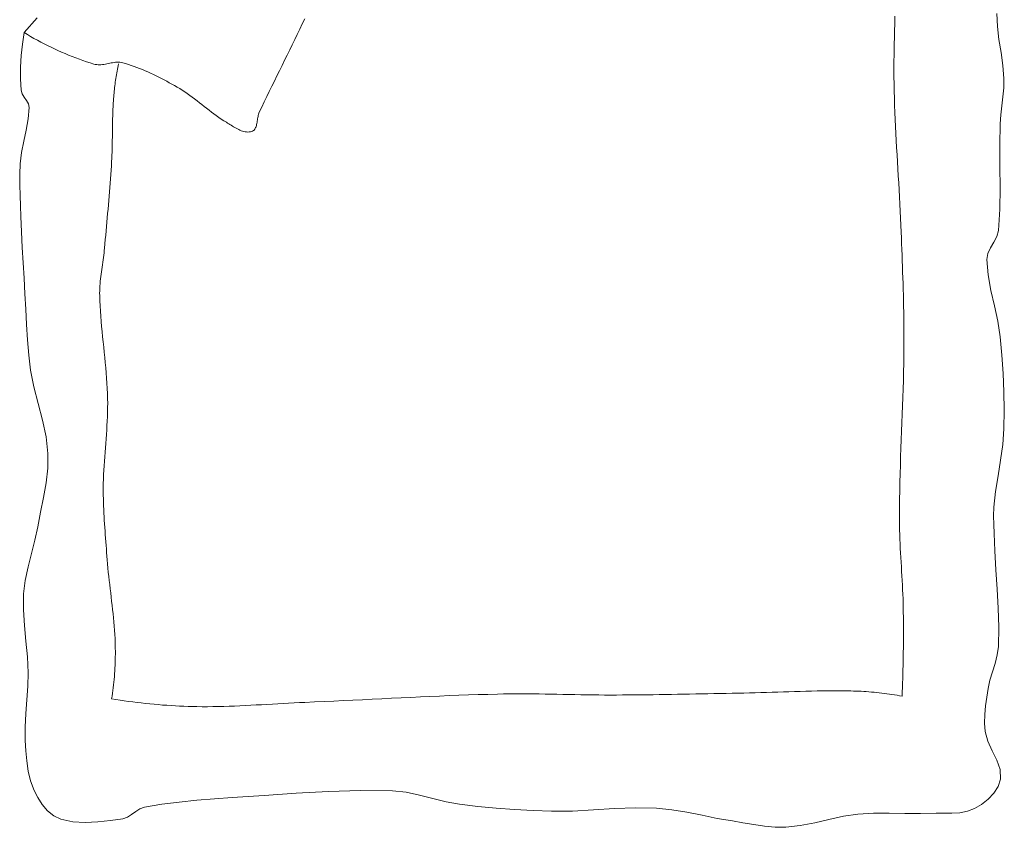
# Model space of a CAD drawing. Units: inches. Extents: x -36302355 to 648, y -221479757 to 75.
# Tile 32 of 37: x 284 to 340, y -66 to -20. Entities that reach past the tile are written whole.
import ezdxf

# ---------------------------------------------------------------- set-up
doc = ezdxf.new("R2010")
doc.units = ezdxf.units.IN
doc.header["$MEASUREMENT"] = 0
doc.layers.add('A-FURN', color=8, linetype='Continuous', lineweight=13)

# ---------------------------------------------------------------- blocks, each defined once
blk = doc.blocks.new('BED-DOUBLE')
for p, q in [((1, 46.159), (0.249, 45.317)), ((16.116, 45.81), (16.256, 46.108)), ((49.913, 45.995), (49.92, 46.246)), ((55.763, 45.66), (55.733, 46.404)), ((15.832, 45.216), (15.975, 45.513)), ((15.975, 45.513), (16.116, 45.81)), ((49.893, 45.241), (49.899, 45.492)), ((49.899, 45.492), (49.906, 45.743)), ((49.906, 45.743), (49.913, 45.995)), ((55.854, 44.918), (55.763, 45.66)), ((0.249, 45.317), (0.154, 44.664)), ((0.249, 45.317), (0.437, 45.204)), ((0.437, 45.204), (0.625, 45.093)), ((0.625, 45.093), (0.815, 44.985)), ((0.815, 44.985), (1.007, 44.879)), ((15.689, 44.919), (15.832, 45.216)), ((49.881, 44.738), (49.887, 44.989)), ((49.887, 44.989), (49.893, 45.241)), ((0.154, 44.664), (0.089, 44.006)), ((1.007, 44.879), (1.2, 44.776)), ((1.2, 44.776), (1.394, 44.675)), ((1.394, 44.675), (1.59, 44.576)), ((1.59, 44.576), (1.787, 44.479)), ((1.787, 44.479), (1.985, 44.386)), ((1.985, 44.386), (2.185, 44.294)), ((15.4, 44.327), (15.545, 44.623)), ((15.545, 44.623), (15.689, 44.919)), ((49.872, 44.235), (49.876, 44.487)), ((49.876, 44.487), (49.881, 44.738)), ((55.971, 44.178), (55.854, 44.918)), ((0.089, 44.006), (0.055, 43.345)), ((2.185, 44.294), (2.385, 44.205)), ((2.385, 44.205), (2.587, 44.119)), ((2.587, 44.119), (2.789, 44.035)), ((2.789, 44.035), (2.993, 43.954)), ((2.993, 43.954), (3.198, 43.875)), ((3.198, 43.875), (3.403, 43.799)), ((15.109, 43.736), (15.255, 44.031)), ((15.255, 44.031), (15.4, 44.327)), ((49.866, 43.733), (49.868, 43.984)), ((49.868, 43.984), (49.872, 44.235)), ((56.076, 43.436), (55.971, 44.178)), ((0.055, 43.345), (0.053, 42.684)), ((3.403, 43.799), (3.609, 43.726)), ((3.609, 43.726), (3.816, 43.655)), ((3.816, 43.655), (4.024, 43.587)), ((4.024, 43.587), (4.233, 43.522)), ((4.233, 43.522), (4.312, 43.502)), ((4.312, 43.502), (4.392, 43.489)), ((4.392, 43.489), (4.473, 43.482)), ((4.473, 43.482), (4.554, 43.482)), ((4.554, 43.482), (4.636, 43.486)), ((4.636, 43.486), (4.719, 43.494)), ((4.719, 43.494), (4.802, 43.505)), ((4.802, 43.505), (4.885, 43.519)), ((4.885, 43.519), (4.969, 43.535)), ((4.969, 43.535), (5.052, 43.552)), ((5.052, 43.552), (5.136, 43.569)), ((5.136, 43.569), (5.22, 43.585)), ((5.22, 43.585), (5.303, 43.599)), ((5.303, 43.599), (5.386, 43.611)), ((5.386, 43.611), (5.469, 43.621)), ((5.469, 43.621), (5.552, 43.626)), ((5.552, 43.626), (5.634, 43.627)), ((5.594, 43.326), (5.575, 43.223)), ((5.615, 43.43), (5.594, 43.326)), ((5.636, 43.533), (5.615, 43.43)), ((5.634, 43.627), (5.715, 43.622)), ((5.715, 43.622), (5.795, 43.611)), ((5.795, 43.611), (5.875, 43.593)), ((5.875, 43.593), (6.038, 43.546)), ((6.038, 43.546), (6.201, 43.496)), ((6.201, 43.496), (6.362, 43.443)), ((6.362, 43.443), (6.523, 43.387)), ((6.523, 43.387), (6.683, 43.329)), ((6.683, 43.329), (6.841, 43.268)), ((6.841, 43.268), (6.999, 43.204)), ((14.817, 43.145), (14.963, 43.44)), ((14.963, 43.44), (15.109, 43.736)), ((49.863, 43.23), (49.864, 43.481)), ((49.864, 43.481), (49.866, 43.733)), ((56.134, 42.692), (56.076, 43.436)), ((0.053, 42.684), (0.081, 42.025)), ((5.486, 42.703), (5.47, 42.599)), ((5.502, 42.808), (5.486, 42.703)), ((5.519, 42.912), (5.502, 42.808)), ((5.537, 43.015), (5.519, 42.912)), ((5.555, 43.119), (5.537, 43.015)), ((5.575, 43.223), (5.555, 43.119)), ((6.999, 43.204), (7.157, 43.138)), ((7.157, 43.138), (7.313, 43.07)), ((7.313, 43.07), (7.468, 43)), ((7.468, 43), (7.623, 42.928)), ((7.623, 42.928), (7.777, 42.854)), ((7.777, 42.854), (7.93, 42.778)), ((7.93, 42.778), (8.082, 42.701)), ((8.082, 42.701), (8.234, 42.622)), ((14.526, 42.554), (14.672, 42.849)), ((14.672, 42.849), (14.817, 43.145)), ((49.863, 42.979), (49.863, 43.23)), ((49.865, 42.727), (49.863, 42.979)), ((49.868, 42.476), (49.865, 42.727)), ((56.124, 42.175), (56.134, 42.692)), ((5.415, 42.181), (5.403, 42.077)), ((5.428, 42.286), (5.415, 42.181)), ((5.441, 42.39), (5.428, 42.286)), ((5.455, 42.495), (5.441, 42.39)), ((5.47, 42.599), (5.455, 42.495)), ((8.234, 42.622), (8.384, 42.542)), ((8.384, 42.542), (8.534, 42.46)), ((8.534, 42.46), (8.683, 42.378)), ((8.683, 42.378), (8.832, 42.295)), ((8.832, 42.295), (8.98, 42.21)), ((8.98, 42.21), (9.128, 42.123)), ((9.128, 42.123), (9.274, 42.031)), ((14.237, 41.962), (14.381, 42.258)), ((14.381, 42.258), (14.526, 42.554)), ((49.872, 42.225), (49.868, 42.476)), ((49.878, 41.973), (49.872, 42.225)), ((56.078, 41.659), (56.124, 42.175)), ((0.081, 42.025), (0.139, 41.819)), ((0.139, 41.819), (0.255, 41.628)), ((0.255, 41.628), (0.387, 41.441)), ((5.362, 41.657), (5.353, 41.552)), ((5.371, 41.762), (5.362, 41.657)), ((5.381, 41.867), (5.371, 41.762)), ((5.392, 41.972), (5.381, 41.867)), ((5.403, 42.077), (5.392, 41.972)), ((9.274, 42.031), (9.418, 41.936)), ((9.418, 41.936), (9.561, 41.838)), ((9.561, 41.838), (9.701, 41.738)), ((9.701, 41.738), (9.84, 41.635)), ((9.84, 41.635), (9.978, 41.531)), ((13.95, 41.369), (14.093, 41.666)), ((14.093, 41.666), (14.237, 41.962)), ((49.889, 41.571), (49.878, 41.973)), ((49.903, 41.169), (49.889, 41.571)), ((56.015, 41.144), (56.078, 41.659)), ((0.387, 41.441), (0.496, 41.249)), ((0.54, 41.043), (0.489, 40.398)), ((0.496, 41.249), (0.54, 41.043)), ((5.325, 41.1), (5.317, 40.926)), ((5.334, 41.274), (5.325, 41.1)), ((5.346, 41.447), (5.334, 41.274)), ((5.353, 41.552), (5.346, 41.447)), ((9.978, 41.531), (10.115, 41.425)), ((10.115, 41.425), (10.252, 41.319)), ((10.252, 41.319), (10.388, 41.212)), ((10.388, 41.212), (10.524, 41.105)), ((10.524, 41.105), (10.661, 40.998)), ((10.661, 40.998), (10.798, 40.892)), ((13.668, 40.774), (13.808, 41.071)), ((13.808, 41.071), (13.95, 41.369)), ((49.918, 40.767), (49.903, 41.169)), ((55.955, 40.628), (56.015, 41.144)), ((5.305, 40.579), (5.301, 40.405)), ((5.311, 40.753), (5.305, 40.579)), ((5.317, 40.926), (5.311, 40.753)), ((10.798, 40.892), (10.935, 40.786)), ((10.935, 40.786), (11.074, 40.683)), ((11.074, 40.683), (11.213, 40.581)), ((11.213, 40.581), (11.354, 40.481)), ((11.354, 40.481), (11.497, 40.385)), ((13.57, 40.401), (13.581, 40.468)), ((13.581, 40.468), (13.594, 40.534)), ((13.594, 40.534), (13.608, 40.598)), ((13.608, 40.598), (13.625, 40.659)), ((13.625, 40.659), (13.645, 40.718)), ((13.645, 40.718), (13.668, 40.774)), ((49.935, 40.364), (49.918, 40.767)), ((55.918, 40.112), (55.955, 40.628)), ((0.489, 40.398), (0.377, 39.758)), ((5.293, 39.883), (5.291, 39.709)), ((5.295, 40.057), (5.293, 39.883)), ((5.298, 40.231), (5.295, 40.057)), ((5.301, 40.405), (5.298, 40.231)), ((11.497, 40.385), (11.642, 40.291)), ((11.642, 40.291), (11.789, 40.201)), ((11.789, 40.201), (11.856, 40.16)), ((11.856, 40.16), (11.923, 40.118)), ((11.923, 40.118), (11.991, 40.075)), ((11.991, 40.075), (12.061, 40.031)), ((12.061, 40.031), (12.131, 39.988)), ((12.131, 39.988), (12.201, 39.944)), ((12.201, 39.944), (12.273, 39.902)), ((12.273, 39.902), (12.345, 39.86)), ((13.433, 39.847), (13.458, 39.897)), ((13.458, 39.897), (13.48, 39.952)), ((13.48, 39.952), (13.498, 40.01)), ((13.498, 40.01), (13.513, 40.071)), ((13.513, 40.071), (13.527, 40.135)), ((13.527, 40.135), (13.539, 40.2)), ((13.539, 40.2), (13.549, 40.267)), ((13.549, 40.267), (13.56, 40.334)), ((13.56, 40.334), (13.57, 40.401)), ((49.954, 39.962), (49.935, 40.364)), ((49.974, 39.56), (49.954, 39.962)), ((55.898, 38.895), (55.918, 40.112)), ((0.377, 39.758), (0.24, 39.119)), ((5.287, 39.361), (5.284, 39.187)), ((5.289, 39.535), (5.287, 39.361)), ((5.291, 39.709), (5.289, 39.535)), ((12.345, 39.86), (12.418, 39.821)), ((12.418, 39.821), (12.491, 39.785)), ((12.491, 39.785), (12.564, 39.752)), ((12.564, 39.752), (12.638, 39.722)), ((12.638, 39.722), (12.712, 39.696)), ((12.712, 39.696), (12.786, 39.675)), ((12.786, 39.675), (12.86, 39.659)), ((12.86, 39.659), (12.934, 39.649)), ((12.934, 39.649), (13.008, 39.646)), ((13.008, 39.646), (13.082, 39.649)), ((13.082, 39.649), (13.156, 39.659)), ((13.156, 39.659), (13.229, 39.677)), ((13.229, 39.677), (13.282, 39.698)), ((13.282, 39.698), (13.328, 39.726)), ((13.328, 39.726), (13.369, 39.761)), ((13.369, 39.761), (13.403, 39.801)), ((13.403, 39.801), (13.433, 39.847)), ((49.996, 39.159), (49.974, 39.56)), ((0.24, 39.119), (0.112, 38.48)), ((5.278, 38.839), (5.274, 38.666)), ((5.282, 39.013), (5.278, 38.839)), ((5.284, 39.187), (5.282, 39.013)), ((50.018, 38.757), (49.996, 39.159)), ((50.04, 38.355), (50.018, 38.757)), ((55.907, 37.677), (55.898, 38.895)), ((0.112, 38.48), (0.028, 37.836)), ((5.262, 38.318), (5.254, 38.144)), ((5.268, 38.492), (5.262, 38.318)), ((5.274, 38.666), (5.268, 38.492)), ((50.064, 37.953), (50.04, 38.355)), ((0.028, 37.836), (0, 37.235)), ((5.229, 37.723), (5.213, 37.476)), ((5.244, 37.971), (5.229, 37.723)), ((5.254, 38.144), (5.244, 37.971)), ((50.087, 37.551), (50.064, 37.953)), ((55.917, 36.459), (55.907, 37.677)), ((0, 37.235), (0, 36.634)), ((5.196, 37.228), (5.178, 36.981)), ((5.213, 37.476), (5.196, 37.228)), ((50.111, 37.149), (50.087, 37.551)), ((50.134, 36.747), (50.111, 37.149)), ((0, 36.634), (0.018, 36.032)), ((5.159, 36.734), (5.14, 36.487)), ((5.178, 36.981), (5.159, 36.734)), ((50.157, 36.345), (50.134, 36.747)), ((0.018, 36.032), (0.045, 35.43)), ((5.1, 35.992), (5.08, 35.745)), ((5.12, 36.239), (5.1, 35.992)), ((5.14, 36.487), (5.12, 36.239)), ((50.179, 35.943), (50.157, 36.345)), ((50.201, 35.542), (50.179, 35.943)), ((55.897, 35.242), (55.917, 36.459)), ((0.045, 35.43), (0.071, 34.828)), ((5.058, 35.498), (5.037, 35.251)), ((5.08, 35.745), (5.058, 35.498)), ((50.222, 35.14), (50.201, 35.542)), ((0.071, 34.828), (0.107, 33.948)), ((5.015, 35.004), (4.993, 34.757)), ((5.037, 35.251), (5.015, 35.004)), ((50.241, 34.737), (50.222, 35.14)), ((55.818, 34.029), (55.897, 35.242)), ((4.949, 34.263), (4.926, 34.016)), ((4.971, 34.51), (4.949, 34.263)), ((4.993, 34.757), (4.971, 34.51)), ((50.259, 34.335), (50.241, 34.737)), ((50.275, 33.933), (50.259, 34.335)), ((0.107, 33.948), (0.149, 33.068)), ((4.904, 33.769), (4.882, 33.522)), ((4.926, 34.016), (4.904, 33.769)), ((50.287, 33.608), (50.275, 33.933)), ((55.726, 33.689), (55.818, 34.029)), ((4.859, 33.275), (4.837, 33.028)), ((4.882, 33.522), (4.859, 33.275)), ((50.3, 33.282), (50.287, 33.608)), ((50.312, 32.957), (50.3, 33.282)), ((55.37, 33.05), (55.558, 33.367)), ((55.558, 33.367), (55.726, 33.689)), ((0.149, 33.068), (0.196, 32.188)), ((4.793, 32.623), (4.776, 32.487)), ((4.809, 32.758), (4.793, 32.623)), ((4.824, 32.893), (4.809, 32.758)), ((4.837, 33.028), (4.824, 32.893)), ((50.325, 32.632), (50.312, 32.957)), ((50.337, 32.306), (50.325, 32.632)), ((55.16, 32.385), (55.219, 32.726)), ((55.219, 32.726), (55.37, 33.05)), ((0.196, 32.188), (0.247, 31.308)), ((4.719, 32.082), (4.7, 31.947)), ((4.739, 32.217), (4.719, 32.082)), ((4.758, 32.352), (4.739, 32.217)), ((4.776, 32.487), (4.758, 32.352)), ((50.348, 31.981), (50.337, 32.306)), ((55.234, 31.495), (55.16, 32.385)), ((4.644, 31.542), (4.627, 31.407)), ((4.662, 31.677), (4.644, 31.542)), ((4.681, 31.812), (4.662, 31.677)), ((4.7, 31.947), (4.681, 31.812)), ((50.36, 31.655), (50.348, 31.981)), ((50.371, 31.33), (50.36, 31.655)), ((55.394, 30.613), (55.234, 31.495)), ((0.247, 31.308), (0.302, 30.429)), ((4.586, 31.001), (4.576, 30.866)), ((4.598, 31.136), (4.586, 31.001)), ((4.612, 31.272), (4.598, 31.136)), ((4.627, 31.407), (4.612, 31.272)), ((50.381, 31.004), (50.371, 31.33)), ((50.39, 30.679), (50.381, 31.004)), ((0.302, 30.429), (0.351, 29.554)), ((4.563, 30.595), (4.561, 30.459)), ((4.561, 30.459), (4.562, 30.323)), ((4.568, 30.73), (4.563, 30.595)), ((4.576, 30.866), (4.568, 30.73)), ((50.399, 30.353), (50.39, 30.679)), ((50.408, 30.028), (50.399, 30.353)), ((55.593, 29.734), (55.394, 30.613)), ((4.562, 30.323), (4.57, 30.028)), ((4.57, 30.028), (4.583, 29.734)), ((50.415, 29.702), (50.408, 30.028)), ((0.351, 29.554), (0.396, 28.679)), ((4.583, 29.734), (4.601, 29.439)), ((4.601, 29.439), (4.621, 29.145)), ((50.421, 29.376), (50.415, 29.702)), ((50.426, 29.051), (50.421, 29.376)), ((55.784, 28.854), (55.593, 29.734)), ((0.396, 28.679), (0.448, 27.804)), ((4.621, 29.145), (4.645, 28.851)), ((4.645, 28.851), (4.671, 28.557)), ((50.43, 28.725), (50.426, 29.051)), ((50.433, 28.4), (50.43, 28.725)), ((55.919, 27.967), (55.784, 28.854)), ((4.671, 28.557), (4.699, 28.263)), ((4.699, 28.263), (4.728, 27.969)), ((50.435, 28.074), (50.433, 28.4)), ((0.448, 27.804), (0.521, 26.932)), ((4.728, 27.969), (4.759, 27.675)), ((4.759, 27.675), (4.79, 27.382)), ((50.434, 27.423), (50.435, 27.749)), ((50.435, 27.749), (50.435, 28.074)), ((56.015, 26.923), (55.919, 27.967)), ((4.79, 27.382), (4.821, 27.088)), ((4.821, 27.088), (4.852, 26.794)), ((50.429, 26.939), (50.434, 27.423)), ((0.521, 26.932), (0.625, 26.063)), ((4.852, 26.794), (4.881, 26.5)), ((4.881, 26.5), (4.909, 26.207)), ((50.412, 25.97), (50.422, 26.454)), ((50.422, 26.454), (50.429, 26.939)), ((56.091, 25.876), (56.015, 26.923)), ((0.625, 26.063), (0.809, 25.109)), ((4.909, 26.207), (4.935, 25.913)), ((4.935, 25.913), (4.958, 25.618)), ((50.399, 25.486), (50.412, 25.97)), ((56.14, 24.828), (56.091, 25.876)), ((4.958, 25.618), (4.978, 25.324)), ((4.978, 25.324), (4.995, 25.03)), ((50.385, 25.001), (50.399, 25.486)), ((0.809, 25.109), (1.05, 24.163)), ((4.995, 25.03), (5.007, 24.735)), ((5.007, 24.735), (5.015, 24.44)), ((50.37, 24.517), (50.385, 25.001)), ((56.158, 23.779), (56.14, 24.828)), ((1.05, 24.163), (1.298, 23.22)), ((5.015, 24.44), (5.018, 24.185)), ((5.018, 24.185), (5.016, 23.931)), ((50.353, 24.033), (50.37, 24.517)), ((5.011, 23.676), (5.002, 23.421)), ((5.016, 23.931), (5.011, 23.676)), ((50.336, 23.549), (50.353, 24.033)), ((56.139, 22.73), (56.158, 23.779)), ((1.298, 23.22), (1.501, 22.271)), ((4.991, 23.166), (4.977, 22.912)), ((5.002, 23.421), (4.991, 23.166)), ((50.299, 22.581), (50.317, 23.065)), ((50.317, 23.065), (50.336, 23.549)), ((4.961, 22.657), (4.943, 22.403)), ((4.977, 22.912), (4.961, 22.657)), ((50.281, 22.096), (50.299, 22.581)), ((56.069, 21.831), (56.139, 22.73)), ((1.501, 22.271), (1.61, 21.31)), ((4.924, 22.148), (4.905, 21.894)), ((4.943, 22.403), (4.924, 22.148)), ((50.263, 21.612), (50.281, 22.096)), ((4.866, 21.385), (4.847, 21.13)), ((4.885, 21.639), (4.866, 21.385)), ((4.905, 21.894), (4.885, 21.639)), ((50.245, 21.128), (50.263, 21.612)), ((55.946, 20.936), (56.069, 21.831)), ((1.61, 21.31), (1.596, 20.47)), ((4.829, 20.876), (4.812, 20.621)), ((4.847, 21.13), (4.829, 20.876)), ((50.229, 20.644), (50.245, 21.128)), ((55.8, 20.042), (55.946, 20.936)), ((1.596, 20.47), (1.501, 19.634)), ((4.798, 20.366), (4.785, 20.111)), ((4.812, 20.621), (4.798, 20.366)), ((50.215, 20.16), (50.229, 20.644)), ((4.776, 19.857), (4.77, 19.602)), ((4.785, 20.111), (4.776, 19.857)), ((50.19, 19.191), (50.201, 19.676)), ((50.201, 19.676), (50.215, 20.16)), ((55.663, 19.148), (55.8, 20.042)), ((1.501, 19.634), (1.355, 18.801)), ((4.77, 19.602), (4.767, 19.347)), ((4.767, 19.347), (4.767, 19.142)), ((4.767, 19.142), (4.77, 18.938)), ((50.182, 18.707), (50.19, 19.191)), ((55.566, 18.25), (55.663, 19.148)), ((1.355, 18.801), (1.187, 17.969)), ((4.77, 18.938), (4.773, 18.733)), ((4.773, 18.733), (4.779, 18.528)), ((50.176, 18.223), (50.182, 18.707)), ((4.779, 18.528), (4.786, 18.323)), ((4.786, 18.323), (4.794, 18.119)), ((4.794, 18.119), (4.803, 17.914)), ((50.173, 17.738), (50.176, 18.223)), ((55.546, 17.754), (55.566, 18.25)), ((1.187, 17.969), (1.029, 17.139)), ((4.803, 17.914), (4.814, 17.71)), ((4.814, 17.71), (4.826, 17.505)), ((4.826, 17.505), (4.838, 17.301)), ((50.174, 17.476), (50.173, 17.738)), ((50.177, 17.214), (50.174, 17.476)), ((55.553, 17.258), (55.546, 17.754)), ((1.029, 17.139), (0.867, 16.371)), ((4.838, 17.301), (4.852, 17.096)), ((4.852, 17.096), (4.866, 16.892)), ((4.866, 16.892), (4.88, 16.688)), ((50.183, 16.952), (50.177, 17.214)), ((50.192, 16.69), (50.183, 16.952)), ((55.576, 16.762), (55.553, 17.258)), ((0.867, 16.371), (0.673, 15.608)), ((4.88, 16.688), (4.895, 16.483)), ((4.895, 16.483), (4.911, 16.279)), ((50.202, 16.429), (50.192, 16.69)), ((50.214, 16.167), (50.202, 16.429)), ((55.604, 16.266), (55.576, 16.762)), ((4.911, 16.279), (4.927, 16.075)), ((4.927, 16.075), (4.943, 15.87)), ((4.943, 15.87), (4.959, 15.666)), ((50.227, 15.905), (50.214, 16.167)), ((50.241, 15.643), (50.227, 15.905)), ((55.626, 15.769), (55.604, 16.266)), ((55.678, 14.678), (55.626, 15.769)), ((0.673, 15.608), (0.479, 14.846)), ((4.959, 15.666), (4.975, 15.462)), ((4.975, 15.462), (4.991, 15.258)), ((4.991, 15.258), (5.01, 15.021)), ((50.256, 15.381), (50.241, 15.643)), ((50.272, 15.12), (50.256, 15.381)), ((0.479, 14.846), (0.317, 14.08)), ((5.01, 15.021), (5.032, 14.784)), ((5.032, 14.784), (5.055, 14.547)), ((50.287, 14.858), (50.272, 15.12)), ((50.303, 14.596), (50.287, 14.858)), ((55.747, 13.587), (55.678, 14.678)), ((0.317, 14.08), (0.222, 13.304)), ((5.055, 14.547), (5.08, 14.31)), ((5.08, 14.31), (5.106, 14.074)), ((5.106, 14.074), (5.133, 13.837)), ((50.319, 14.334), (50.303, 14.596)), ((50.333, 14.073), (50.319, 14.334)), ((50.347, 13.811), (50.333, 14.073)), ((5.133, 13.837), (5.161, 13.601)), ((5.161, 13.601), (5.189, 13.364)), ((50.36, 13.549), (50.347, 13.811)), ((50.371, 13.287), (50.36, 13.549)), ((55.809, 12.496), (55.747, 13.587)), ((0.222, 13.304), (0.211, 12.406)), ((5.189, 13.364), (5.218, 13.128)), ((5.218, 13.128), (5.246, 12.892)), ((50.381, 13.025), (50.371, 13.287)), ((50.388, 12.763), (50.381, 13.025)), ((0.211, 12.406), (0.269, 11.508)), ((5.246, 12.892), (5.273, 12.655)), ((5.273, 12.655), (5.3, 12.419)), ((5.3, 12.419), (5.325, 12.182)), ((50.394, 12.501), (50.388, 12.763)), ((50.397, 12.25), (50.394, 12.501)), ((55.842, 11.405), (55.809, 12.496)), ((5.325, 12.182), (5.349, 11.946)), ((5.349, 11.946), (5.372, 11.709)), ((50.4, 11.999), (50.397, 12.25)), ((50.402, 11.747), (50.4, 11.999)), ((0.269, 11.508), (0.358, 10.61)), ((5.372, 11.709), (5.392, 11.472)), ((5.392, 11.472), (5.41, 11.235)), ((5.41, 11.235), (5.425, 10.998)), ((50.403, 11.496), (50.402, 11.747)), ((50.404, 11.244), (50.403, 11.496)), ((50.404, 10.993), (50.404, 11.244)), ((55.821, 10.315), (55.842, 11.405)), ((5.425, 10.998), (5.438, 10.76)), ((5.438, 10.76), (5.447, 10.523)), ((50.402, 10.49), (50.403, 10.742)), ((50.403, 10.742), (50.404, 10.993)), ((0.358, 10.61), (0.444, 9.712)), ((5.447, 10.523), (5.452, 10.363)), ((5.452, 10.363), (5.454, 10.202)), ((5.454, 10.202), (5.456, 10.042)), ((50.397, 9.987), (50.4, 10.239)), ((50.4, 10.239), (50.402, 10.49)), ((55.755, 9.827), (55.821, 10.315)), ((0.444, 9.712), (0.487, 8.812)), ((5.451, 9.56), (5.446, 9.399)), ((5.454, 9.721), (5.451, 9.56)), ((5.456, 9.881), (5.454, 9.721)), ((5.456, 10.042), (5.456, 9.881)), ((50.389, 9.485), (50.393, 9.736)), ((50.393, 9.736), (50.397, 9.987)), ((55.631, 9.348), (55.755, 9.827)), ((5.432, 9.078), (5.422, 8.918)), ((5.44, 9.239), (5.432, 9.078)), ((5.446, 9.399), (5.44, 9.239)), ((50.379, 8.982), (50.384, 9.233)), ((50.384, 9.233), (50.389, 9.485)), ((55.479, 8.873), (55.631, 9.348)), ((0.487, 8.812), (0.469, 8.039)), ((5.385, 8.437), (5.37, 8.278)), ((5.399, 8.598), (5.385, 8.437)), ((5.412, 8.758), (5.399, 8.598)), ((5.422, 8.918), (5.412, 8.758)), ((50.357, 8.228), (50.365, 8.479)), ((50.365, 8.479), (50.372, 8.731)), ((50.372, 8.731), (50.379, 8.982)), ((55.334, 8.396), (55.479, 8.873)), ((0.469, 8.039), (0.415, 7.265)), ((5.335, 7.958), (5.315, 7.799)), ((5.353, 8.118), (5.335, 7.958)), ((5.37, 8.278), (5.353, 8.118)), ((50.34, 7.726), (50.349, 7.977)), ((50.349, 7.977), (50.357, 8.228)), ((55.153, 7.423), (55.228, 7.912)), ((55.228, 7.912), (55.334, 8.396)), ((5.27, 7.481), (5.246, 7.323)), ((5.246, 7.323), (5.486, 7.284)), ((5.293, 7.64), (5.27, 7.481)), ((5.315, 7.799), (5.293, 7.64)), ((19.558, 7.278), (20.107, 7.305)), ((20.107, 7.305), (20.656, 7.332)), ((20.656, 7.332), (21.206, 7.359)), ((21.206, 7.359), (21.755, 7.385)), ((21.755, 7.385), (22.304, 7.411)), ((22.304, 7.411), (22.853, 7.436)), ((22.853, 7.436), (23.402, 7.461)), ((23.402, 7.461), (23.952, 7.484)), ((23.952, 7.484), (24.501, 7.507)), ((24.501, 7.507), (25.05, 7.528)), ((25.05, 7.528), (25.6, 7.547)), ((25.6, 7.547), (26.149, 7.565)), ((26.149, 7.565), (26.698, 7.581)), ((26.698, 7.581), (27.248, 7.595)), ((27.248, 7.595), (27.588, 7.602)), ((27.588, 7.602), (27.927, 7.606)), ((27.927, 7.606), (28.267, 7.609)), ((28.267, 7.609), (28.607, 7.609)), ((28.607, 7.609), (28.946, 7.608)), ((28.946, 7.608), (29.286, 7.605)), ((29.286, 7.605), (29.626, 7.602)), ((29.626, 7.602), (29.966, 7.597)), ((29.966, 7.597), (30.305, 7.592)), ((30.305, 7.592), (30.645, 7.586)), ((30.645, 7.586), (30.985, 7.579)), ((30.985, 7.579), (31.325, 7.573)), ((31.325, 7.573), (31.664, 7.566)), ((31.664, 7.566), (32.004, 7.56)), ((32.004, 7.56), (32.344, 7.555)), ((32.344, 7.555), (32.684, 7.55)), ((32.684, 7.55), (33.023, 7.546)), ((33.023, 7.546), (33.363, 7.544)), ((33.363, 7.544), (33.703, 7.543)), ((33.703, 7.543), (34.043, 7.543)), ((34.043, 7.543), (34.39, 7.545)), ((34.39, 7.545), (34.737, 7.547)), ((34.737, 7.547), (35.085, 7.55)), ((35.085, 7.55), (35.432, 7.554)), ((35.432, 7.554), (35.779, 7.558)), ((35.779, 7.558), (36.127, 7.563)), ((36.127, 7.563), (36.474, 7.568)), ((36.474, 7.568), (36.821, 7.573)), ((36.821, 7.573), (37.168, 7.579)), ((37.168, 7.579), (37.516, 7.585)), ((37.516, 7.585), (37.863, 7.591)), ((37.863, 7.591), (38.21, 7.598)), ((38.21, 7.598), (38.558, 7.604)), ((38.558, 7.604), (38.905, 7.611)), ((38.905, 7.611), (39.252, 7.618)), ((39.252, 7.618), (39.599, 7.625)), ((39.599, 7.625), (39.947, 7.631)), ((39.947, 7.631), (40.294, 7.638)), ((40.294, 7.638), (40.641, 7.644)), ((40.641, 7.644), (40.989, 7.65)), ((40.989, 7.65), (41.309, 7.657)), ((41.309, 7.657), (41.63, 7.664)), ((41.63, 7.664), (41.951, 7.672)), ((41.951, 7.672), (42.272, 7.681)), ((42.272, 7.681), (42.593, 7.691)), ((42.593, 7.691), (42.914, 7.701)), ((42.914, 7.701), (43.235, 7.712)), ((43.235, 7.712), (43.556, 7.722)), ((43.556, 7.722), (43.877, 7.732)), ((43.877, 7.732), (44.198, 7.742)), ((44.198, 7.742), (44.519, 7.751)), ((44.519, 7.751), (44.839, 7.76)), ((44.839, 7.76), (45.16, 7.767)), ((45.16, 7.767), (45.481, 7.773)), ((45.481, 7.773), (45.802, 7.778)), ((45.802, 7.778), (46.123, 7.782)), ((46.123, 7.782), (46.444, 7.783)), ((46.444, 7.783), (46.765, 7.783)), ((46.765, 7.783), (47.086, 7.78)), ((47.086, 7.78), (47.407, 7.776)), ((47.407, 7.776), (47.554, 7.772)), ((47.554, 7.772), (47.701, 7.768)), ((47.701, 7.768), (47.847, 7.762)), ((47.847, 7.762), (47.994, 7.755)), ((47.994, 7.755), (48.141, 7.746)), ((48.141, 7.746), (48.288, 7.737)), ((48.288, 7.737), (48.435, 7.726)), ((48.435, 7.726), (48.582, 7.714)), ((48.582, 7.714), (48.728, 7.701)), ((48.728, 7.701), (48.875, 7.686)), ((48.875, 7.686), (49.021, 7.671)), ((49.021, 7.671), (49.167, 7.654)), ((49.167, 7.654), (49.313, 7.635)), ((49.313, 7.635), (49.459, 7.616)), ((49.459, 7.616), (49.605, 7.596)), ((49.605, 7.596), (49.75, 7.574)), ((49.75, 7.574), (49.896, 7.551)), ((49.896, 7.551), (50.041, 7.527)), ((50.041, 7.527), (50.185, 7.501)), ((50.185, 7.501), (50.33, 7.475)), ((50.33, 7.475), (50.34, 7.726)), ((55.086, 6.932), (55.153, 7.423)), ((0.415, 7.265), (0.354, 6.492)), ((5.486, 7.284), (5.727, 7.247)), ((5.727, 7.247), (5.968, 7.212)), ((5.968, 7.212), (6.21, 7.179)), ((6.21, 7.179), (6.451, 7.147)), ((6.451, 7.147), (6.693, 7.117)), ((6.693, 7.117), (6.935, 7.089)), ((6.935, 7.089), (7.178, 7.062)), ((7.178, 7.062), (7.42, 7.038)), ((7.42, 7.038), (7.663, 7.015)), ((7.663, 7.015), (7.906, 6.994)), ((7.906, 6.994), (8.149, 6.974)), ((8.149, 6.974), (8.392, 6.956)), ((8.392, 6.956), (8.635, 6.941)), ((8.635, 6.941), (8.879, 6.927)), ((8.879, 6.927), (9.122, 6.914)), ((9.122, 6.914), (9.365, 6.904)), ((9.365, 6.904), (9.609, 6.895)), ((9.609, 6.895), (9.852, 6.888)), ((9.852, 6.888), (10.096, 6.883)), ((10.096, 6.883), (10.404, 6.879)), ((10.404, 6.879), (10.713, 6.878)), ((10.713, 6.878), (11.021, 6.88)), ((11.021, 6.88), (11.33, 6.886)), ((11.33, 6.886), (11.638, 6.893)), ((11.638, 6.893), (11.947, 6.903)), ((11.947, 6.903), (12.255, 6.914)), ((12.255, 6.914), (12.563, 6.928)), ((12.563, 6.928), (12.872, 6.942)), ((12.872, 6.942), (13.18, 6.958)), ((13.18, 6.958), (13.488, 6.975)), ((13.488, 6.975), (13.796, 6.993)), ((13.796, 6.993), (14.105, 7.011)), ((14.105, 7.011), (14.413, 7.029)), ((14.413, 7.029), (14.721, 7.047)), ((14.721, 7.047), (15.03, 7.064)), ((15.03, 7.064), (15.338, 7.081)), ((15.338, 7.081), (15.646, 7.097)), ((15.646, 7.097), (15.955, 7.112)), ((15.955, 7.112), (16.263, 7.126)), ((16.263, 7.126), (16.812, 7.149)), ((16.812, 7.149), (17.361, 7.174)), ((17.361, 7.174), (17.911, 7.199)), ((17.911, 7.199), (18.46, 7.225)), ((18.46, 7.225), (19.009, 7.251)), ((19.009, 7.251), (19.558, 7.278)), ((55.042, 6.439), (55.086, 6.932)), ((0.354, 6.492), (0.312, 5.719)), ((55.032, 5.947), (55.042, 6.439)), ((0.312, 5.719), (0.317, 4.946)), ((55.071, 5.457), (55.032, 5.947)), ((55.224, 4.905), (55.071, 5.457)), ((0.317, 4.946), (0.35, 4.366)), ((55.472, 4.369), (55.224, 4.905)), ((0.35, 4.366), (0.401, 3.783)), ((55.73, 3.838), (55.472, 4.369)), ((0.401, 3.783), (0.486, 3.207)), ((55.915, 3.301), (55.73, 3.838)), ((0.486, 3.207), (0.62, 2.644)), ((55.943, 2.749), (55.915, 3.301)), ((0.62, 2.644), (0.821, 2.105)), ((55.568, 1.939), (55.814, 2.324)), ((55.814, 2.324), (55.943, 2.749)), ((0.821, 2.105), (1.03, 1.695)), ((1.03, 1.695), (1.287, 1.3)), ((11.115, 1.628), (12.122, 1.697)), ((12.122, 1.697), (13.949, 1.822)), ((13.949, 1.822), (15.777, 1.943)), ((15.777, 1.943), (17.605, 2.039)), ((17.605, 2.039), (19.435, 2.09)), ((19.435, 2.09), (21.264, 2.075)), ((21.264, 2.075), (22.035, 1.997)), ((22.035, 1.997), (22.798, 1.838)), ((22.798, 1.838), (23.556, 1.643)), ((55.24, 1.598), (55.568, 1.939)), ((1.287, 1.3), (1.593, 0.945)), ((6.853, 1.046), (7.11, 1.141)), ((7.11, 1.141), (8.104, 1.311)), ((8.104, 1.311), (9.104, 1.443)), ((9.104, 1.443), (10.109, 1.546)), ((10.109, 1.546), (11.115, 1.628)), ((23.556, 1.643), (24.315, 1.453)), ((24.315, 1.453), (25.082, 1.315)), ((25.082, 1.315), (26.129, 1.191)), ((26.129, 1.191), (27.178, 1.088)), ((54.464, 1.069), (54.861, 1.307)), ((54.861, 1.307), (55.24, 1.598)), ((1.593, 0.945), (1.947, 0.659)), ((1.947, 0.659), (2.35, 0.467)), ((5.885, 0.491), (6.145, 0.575)), ((6.145, 0.575), (6.384, 0.722)), ((6.384, 0.722), (6.615, 0.893)), ((6.615, 0.893), (6.853, 1.046)), ((27.178, 1.088), (28.229, 1.007)), ((28.229, 1.007), (29.281, 0.949)), ((29.281, 0.949), (30.334, 0.915)), ((30.334, 0.915), (31.531, 0.929)), ((31.531, 0.929), (32.728, 0.991)), ((32.728, 0.991), (33.925, 1.065)), ((33.925, 1.065), (35.121, 1.111)), ((35.121, 1.111), (36.317, 1.092)), ((36.317, 1.092), (37.189, 1.006)), ((37.189, 1.006), (38.055, 0.862)), ((38.055, 0.862), (38.918, 0.688)), ((38.918, 0.688), (39.781, 0.511)), ((46.158, 0.453), (46.977, 0.631)), ((46.977, 0.631), (47.803, 0.751)), ((47.803, 0.751), (48.694, 0.802)), ((48.694, 0.802), (49.587, 0.807)), ((49.587, 0.807), (50.481, 0.791)), ((50.481, 0.791), (51.375, 0.779)), ((51.375, 0.779), (52.268, 0.798)), ((52.268, 0.798), (52.717, 0.807)), ((52.717, 0.807), (53.172, 0.809)), ((53.172, 0.809), (53.622, 0.834)), ((53.622, 0.834), (54.056, 0.911)), ((54.056, 0.911), (54.464, 1.069)), ((2.35, 0.467), (3.037, 0.316)), ((3.037, 0.316), (3.743, 0.273)), ((3.743, 0.273), (4.46, 0.308)), ((4.46, 0.308), (5.177, 0.39)), ((5.177, 0.39), (5.885, 0.491)), ((39.781, 0.511), (40.647, 0.36)), ((40.647, 0.36), (41.254, 0.26)), ((41.254, 0.26), (41.863, 0.152)), ((41.863, 0.152), (42.472, 0.059)), ((42.472, 0.059), (43.083, 0.002)), ((43.083, 0.002), (43.695, 0)), ((43.695, 0), (44.523, 0.095)), ((44.523, 0.095), (45.342, 0.26)), ((45.342, 0.26), (46.158, 0.453))]:
    blk.add_line(p, q)

msp = doc.modelspace()

# ---------------------------------------------------------------- block references
at = {"layer": 'A-FURN'}
msp.add_blockref('BED-DOUBLE', (283.833, -65.73), dxfattribs=at)

doc.saveas('drawing.dxf')
